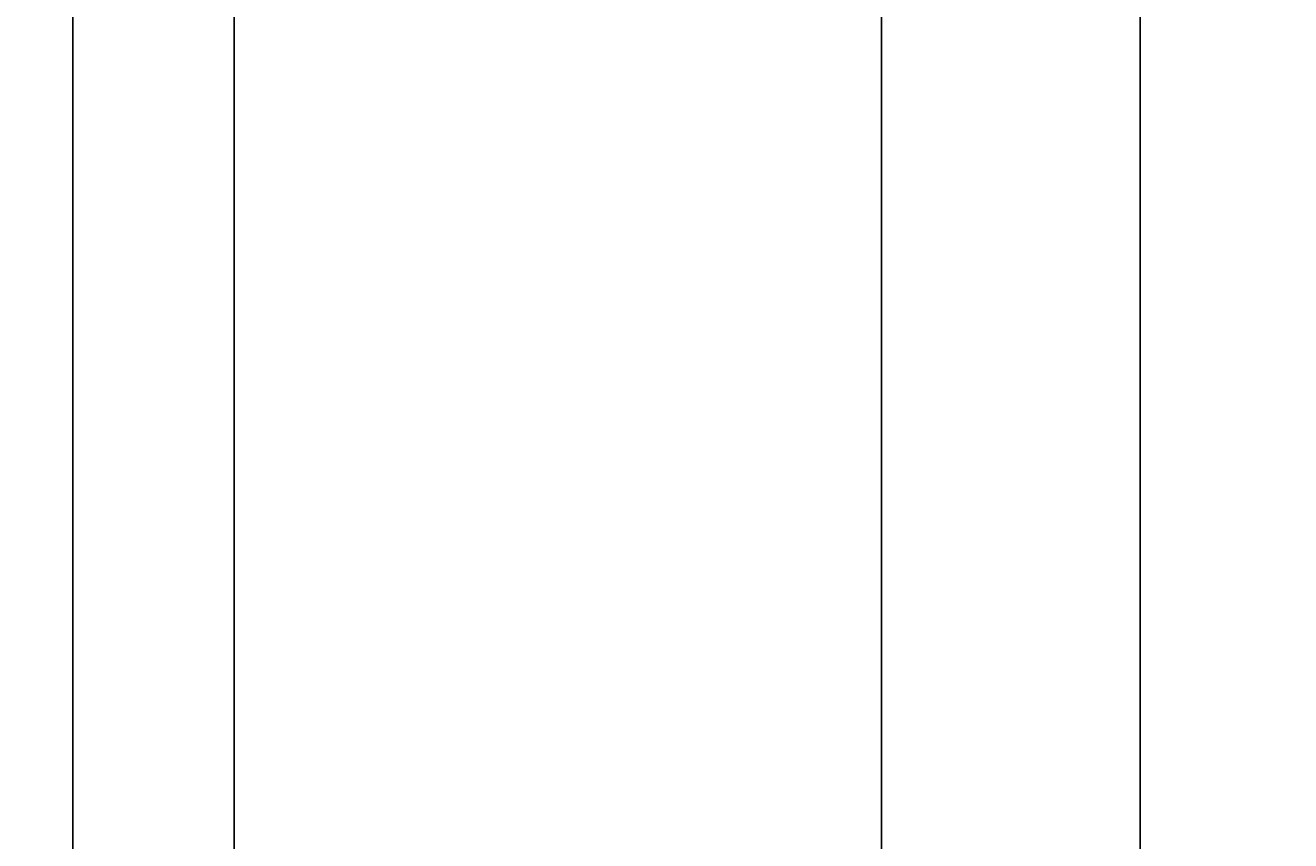
# Model space of a CAD drawing. Units: inches. Extents: x 738 to 1068, y 378 to 757.
# Tile 14 of 41: x 882 to 911, y 417 to 435. Entities that reach past the tile are written whole.
import ezdxf

# ---------------------------------------------------------------- set-up
doc = ezdxf.new("R2010")
doc.units = ezdxf.units.IN
doc.header["$MEASUREMENT"] = 0
doc.layers.add('A-ANNO-DIMS', color=2, linetype='Continuous', lineweight=18)
doc.styles.get("Standard").update_dxf_attribs({"font": 'arial.ttf'})
doc.dimstyles.get("Standard").update_dxf_attribs({"dimtxt": 0.18, "dimasz": 0.18, "dimexe": 0.18, "dimexo": 0.0625, "dimgap": 0.09, "dimtad": 0, "dimtih": 1, "dimtoh": 1, "dimdec": 4, "dimzin": 0, "dimdsep": 46, "dimtxsty": 'Standard', "dimcen": 0.09, "dimadec": 0, "dimazin": 0, "dimtfac": 1, "dimtdec": 4, "dimtofl": 0, "dimtmove": 0, "dimatfit": 3, "dimfxl": 1, "dimtolj": 1, "dimtzin": 0, "dimarcsym": 0})

# ---------------------------------------------------------------- blocks, each defined once
blk = doc.blocks.new('*D18')
at = {"layer": 'A-ANNO-DIMS', "color": 0, "lineweight": -2, "transparency": 16777216}
for p, q in [((901.525, 738.375), (1068.179, 738.375)), ((1067.999, 738.195), (1067.999, 569.167)), ((1067.999, 399.775), (1067.999, 568.803)), ((1023.842, 399.595), (1068.179, 399.595))]:
    blk.add_line(p, q, dxfattribs=at)
at = {"layer": 'A-ANNO-DIMS', "color": 0, "transparency": 16777216}
for points in [[(1067.969, 738.195), (1068.029, 738.195), (1067.999, 738.375)], [(1067.969, 399.775), (1068.029, 399.775), (1067.999, 399.595)]]:
    blk.add_solid(points, dxfattribs=at)
at = {"layer": 'Defpoints', "color": 0, "transparency": 16777216}
for p in [(901.462, 738.375), (1067.999, 738.375), (1023.779, 399.595)]:
    blk.add_point(p, dxfattribs=at)
at = {"layer": 'A-ANNO-DIMS', "color": 0, "transparency": 16777216, "insert": (1067.999, 568.985), "char_height": 0.18, "attachment_point": 5}
blk.add_mtext('\\A1;338.8', dxfattribs=at)
blk = doc.blocks.new('*D27')
at = {"layer": 'A-ANNO-DIMS', "color": 0, "lineweight": -2, "transparency": 16777216}
for p, q in [((883.457, 646.923), (883.457, 378.239)), ((923.511, 646.923), (923.511, 378.239)), ((883.637, 378.419), (903.086, 378.419)), ((923.331, 378.419), (903.882, 378.419))]:
    blk.add_line(p, q, dxfattribs=at)
at = {"layer": 'A-ANNO-DIMS', "color": 0, "transparency": 16777216}
for points in [[(883.637, 378.449), (883.637, 378.389), (883.457, 378.419)], [(923.331, 378.449), (923.331, 378.389), (923.511, 378.419)]]:
    blk.add_solid(points, dxfattribs=at)
at = {"layer": 'Defpoints', "color": 0, "transparency": 16777216}
for p in [(883.457, 646.985), (923.511, 646.985), (923.511, 378.419)]:
    blk.add_point(p, dxfattribs=at)
at = {"layer": 'A-ANNO-DIMS', "color": 0, "transparency": 16777216, "insert": (903.484, 378.419), "char_height": 0.18, "attachment_point": 5}
blk.add_mtext('\\A1;40.05', dxfattribs=at)
blk = doc.blocks.new('*D33')
at = {"layer": 'A-ANNO-DIMS', "color": 0, "lineweight": -2, "transparency": 16777216}
for p, q in [((836.324, 514.624), (836.324, 378.239)), ((907.171, 514.624), (907.171, 378.239)), ((836.504, 378.419), (871.354, 378.419)), ((906.991, 378.419), (872.141, 378.419))]:
    blk.add_line(p, q, dxfattribs=at)
at = {"layer": 'A-ANNO-DIMS', "color": 0, "transparency": 16777216}
for points in [[(836.504, 378.449), (836.504, 378.389), (836.324, 378.419)], [(906.991, 378.449), (906.991, 378.389), (907.171, 378.419)]]:
    blk.add_solid(points, dxfattribs=at)
at = {"layer": 'Defpoints', "color": 0, "transparency": 16777216}
for p in [(836.324, 514.687), (907.171, 514.687), (907.171, 378.419)]:
    blk.add_point(p, dxfattribs=at)
at = {"layer": 'A-ANNO-DIMS', "color": 0, "transparency": 16777216, "insert": (871.748, 378.419), "char_height": 0.18, "attachment_point": 5}
blk.add_mtext('\\A1;70.85', dxfattribs=at)
blk = doc.blocks.new('*D35')
at = {"layer": 'A-ANNO-DIMS', "color": 0, "lineweight": -2, "transparency": 16777216}
for p, q in [((855.932, 686.266), (855.932, 378.239)), ((901.429, 686.267), (901.429, 378.239)), ((856.112, 378.419), (878.352, 378.419)), ((901.249, 378.419), (879.009, 378.419))]:
    blk.add_line(p, q, dxfattribs=at)
at = {"layer": 'A-ANNO-DIMS', "color": 0, "transparency": 16777216}
for points in [[(856.112, 378.449), (856.112, 378.389), (855.932, 378.419)], [(901.249, 378.449), (901.249, 378.389), (901.429, 378.419)]]:
    blk.add_solid(points, dxfattribs=at)
at = {"layer": 'Defpoints', "color": 0, "transparency": 16777216}
for p in [(855.932, 686.329), (901.429, 686.329), (901.429, 378.419)]:
    blk.add_point(p, dxfattribs=at)
at = {"layer": 'A-ANNO-DIMS', "color": 0, "transparency": 16777216, "insert": (878.68, 378.419), "char_height": 0.18, "attachment_point": 5}
blk.add_mtext('\\A1;45.5', dxfattribs=at)
blk = doc.blocks.new('*D38')
at = {"layer": 'A-ANNO-DIMS', "color": 0, "lineweight": -2, "transparency": 16777216}
for p, q in [((781.485, 593.017), (781.485, 378.239)), ((887.04, 593.067), (887.04, 378.239)), ((781.665, 378.419), (833.807, 378.419)), ((886.86, 378.419), (834.718, 378.419))]:
    blk.add_line(p, q, dxfattribs=at)
at = {"layer": 'A-ANNO-DIMS', "color": 0, "transparency": 16777216}
for points in [[(781.665, 378.449), (781.665, 378.389), (781.485, 378.419)], [(886.86, 378.449), (886.86, 378.389), (887.04, 378.419)]]:
    blk.add_solid(points, dxfattribs=at)
at = {"layer": 'Defpoints', "color": 0, "transparency": 16777216}
for p in [(887.04, 593.13), (781.485, 593.08), (887.04, 378.419)]:
    blk.add_point(p, dxfattribs=at)
at = {"layer": 'A-ANNO-DIMS', "color": 0, "transparency": 16777216, "insert": (834.263, 378.419), "char_height": 0.18, "attachment_point": 5}
blk.add_mtext('\\A1;105.56', dxfattribs=at)
blk = doc.blocks.new('*D39')
at = {"layer": 'A-ANNO-DIMS', "color": 0, "lineweight": -2, "transparency": 16777216}
for p, q in [((887.04, 581.418), (887.04, 378.239)), ((938.455, 581.418), (938.455, 378.239)), ((887.22, 378.419), (912.371, 378.419)), ((938.275, 378.419), (913.124, 378.419))]:
    blk.add_line(p, q, dxfattribs=at)
at = {"layer": 'A-ANNO-DIMS', "color": 0, "transparency": 16777216}
for points in [[(887.22, 378.449), (887.22, 378.389), (887.04, 378.419)], [(938.275, 378.449), (938.275, 378.389), (938.455, 378.419)]]:
    blk.add_solid(points, dxfattribs=at)
at = {"layer": 'Defpoints', "color": 0, "transparency": 16777216}
for p in [(887.04, 581.481), (938.455, 581.481), (938.455, 378.419)]:
    blk.add_point(p, dxfattribs=at)
at = {"layer": 'A-ANNO-DIMS', "color": 0, "transparency": 16777216, "insert": (912.748, 378.419), "char_height": 0.18, "attachment_point": 5}
blk.add_mtext('\\A1;51.41', dxfattribs=at)

msp = doc.modelspace()

# ---------------------------------------------------------------- dimensions: what is measured, and where the dimension line sits
at = {"layer": 'A-ANNO-DIMS'}
dim = msp.add_linear_dim(base=(1067.9992, 738.3751), p1=(1023.779, 399.5952), p2=(901.4622, 738.3751), angle=90, dimstyle='Standard', override={"dimdec": 1, "dimlfac": 1, "dimrnd": 0, "dimzin": 0, "dimdsep": 46, "dimlunit": 2}, dxfattribs=at)
dim.commit()
dim.dimension.update_dxf_attribs({"geometry": '*D18', "text_midpoint": (1067.9992, 568.9851)})
for base, p1, p2, override, picture, middle in [((901.4286, 378.4191), (855.9323, 686.329), (901.4286, 686.3292), {"dimdec": 1, "dimlfac": 1, "dimrnd": 0, "dimzin": 0, "dimdsep": 46, "dimlunit": 2}, '*D35', (878.6804, 378.4191)), ((923.5105, 378.4191), (883.4574, 646.9853), (923.5105, 646.9853), {"dimdec": 2, "dimlfac": 1, "dimrnd": 0, "dimzin": 0, "dimdsep": 46, "dimlunit": 2}, '*D27', (903.484, 378.4191)), ((887.0404, 378.4191), (781.4846, 593.0796), (887.0404, 593.1296), {"dimdec": 2, "dimlfac": 1, "dimrnd": 0, "dimzin": 0, "dimdsep": 46, "dimlunit": 2}, '*D38', (834.2625, 378.4191)), ((938.455, 378.4191), (887.0404, 581.4808), (938.455, 581.4808), {"dimdec": 2, "dimlfac": 1, "dimrnd": 0, "dimzin": 0, "dimdsep": 46, "dimlunit": 2}, '*D39', (912.7477, 378.4191)), ((907.1708, 378.4191), (836.3244, 514.6866), (907.1708, 514.6866), {"dimdec": 2, "dimlfac": 1, "dimrnd": 0, "dimzin": 0, "dimdsep": 46, "dimlunit": 2}, '*D33', (871.7476, 378.4191))]:
    dim = msp.add_linear_dim(base=base, p1=p1, p2=p2, dimstyle='Standard', override=override, dxfattribs=at)
    dim.commit()
    dim.dimension.update_dxf_attribs({"geometry": picture, "text_midpoint": middle})

doc.saveas('drawing.dxf')
